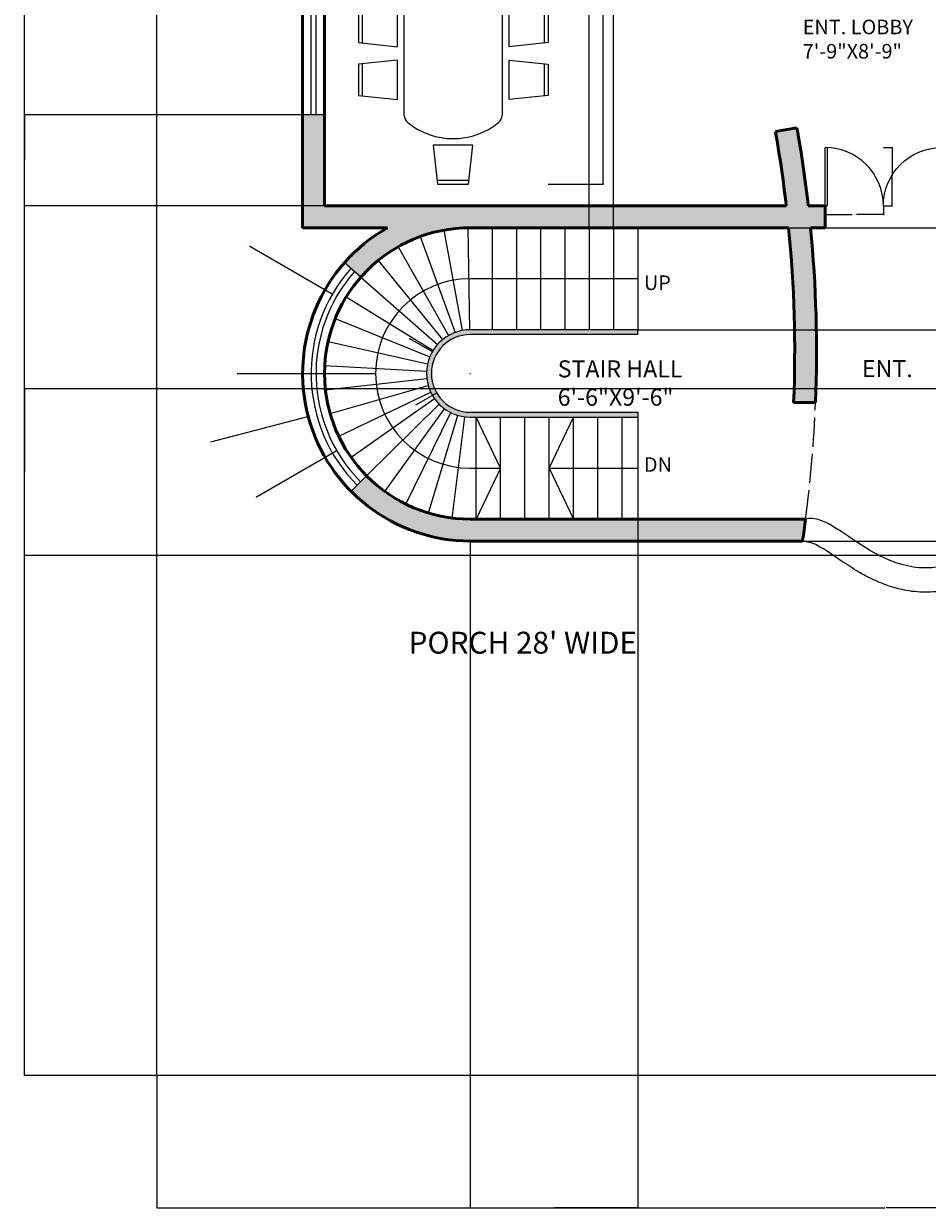
# Model space of a CAD drawing. Units: inches. Extents: x 134045 to 134755, y 144691 to 145880.
# Tile 1 of 6: x 134045 to 134417, y 144691 to 145178. Entities that reach past the tile are written whole.
import ezdxf

# ---------------------------------------------------------------- set-up
doc = ezdxf.new("R2010")
doc.units = ezdxf.units.IN
doc.linetypes.add('ACAD_ISO02W100', pattern=[15, 12, -3])
for name, color, linetype, lineweight in [('A-ANNO-DIMS', 2, 'Continuous', 18), ('A-ANNO-SYMB', 7, 'Continuous', 18), ('A-ANNO-TEXT', 7, 'Continuous', 18), ('A-AREA-IDEN', 7, 'Continuous', 18), ('A-DOOR', 4, 'Continuous', 25), ('A-FLOR-STEP', 7, 'Continuous', 25), ('A-FLOR-STRS', 7, 'Continuous', 25), ('A-FLOR-STRS-PATT', 252, 'Continuous', 13), ('A-FURN', 8, 'Continuous', 18), ('A-GLAZ', 4, 'Continuous', 18), ('A-WALL', 7, 'Continuous', 50), ('A-WALL-OVHD', 7, 'ACAD_ISO02W100', 18), ('A-WALL-PATT', 252, 'Continuous', 13), ('C-PROP', 7, 'Continuous', 25)]:
    doc.layers.add(name, color=color, linetype=linetype, lineweight=lineweight)
doc.styles.get("Standard").update_dxf_attribs({"font": 'arial.ttf'})
doc.dimstyles.get("Standard").update_dxf_attribs({"dimtxt": 0.18, "dimasz": 0.18, "dimexe": 0.18, "dimexo": 0.0625, "dimgap": 0.09, "dimtad": 0, "dimtih": 1, "dimtoh": 1, "dimdec": 4, "dimzin": 0, "dimdsep": 46, "dimtxsty": 'Standard', "dimcen": 0.09, "dimadec": 0, "dimazin": 0, "dimtfac": 1, "dimtdec": 4, "dimtofl": 0, "dimtmove": 0, "dimatfit": 3, "dimfxl": 1, "dimtolj": 1, "dimtzin": 0, "dimarcsym": 0})

# ---------------------------------------------------------------- blocks, each defined once
blk = doc.blocks.new('*U1')
blk.add_line((0, 0), (0, 42))
blk = doc.blocks.new('*U2')
at = {"layer": 'A-FLOR-STRS', "color": 0, "linetype": 'ByBlock', "lineweight": -2, "transparency": 16777216}
for p, rotation in [((134208.53, 145090.74), 200.0535228295788), ((134218.17, 145093.37), 190.5042262440651), ((134228.1, 145094.37), 180.9549296585513), ((134238.1, 145094.38), 180), ((134248.1, 145094.38), 180), ((134258.1, 145094.38), 180), ((134268.1, 145094.38), 180), ((134278.1, 145094.38), 180), ((134288.1, 145094.38), 180), ((134298.1, 145094.38), 180), ((134199.46, 145086.54), 209.6028194150926), ((134191.22, 145080.9), 219.1521160006063), ((134184.03, 145073.97), 228.70141258612), ((134178.08, 145065.95), 238.2507091716337), ((134173.55, 145057.05), 247.8000057571474), ((134170.56, 145047.52), 257.3493023426611), ((134169.19, 145037.62), 266.8985989281748), ((134169.48, 145027.64), 276.4478955136885), ((134171.43, 145017.84), 285.9971920992022), ((134174.97, 145008.5), 295.5464886847159), ((134180.01, 144999.88), 305.0957852702297), ((134186.42, 144992.21), 314.6450818557434), ((134194, 144985.71), 324.1943784412572), ((134202.56, 144980.57), 333.7436750267709), ((134211.86, 144976.91), 343.2929716122846), ((134221.63, 144974.84), 352.8422681977984)]:
    blk.add_blockref('*U1', p, dxfattribs=dict(at, rotation=rotation))
for p in [(134231.61, 144974.38), (134241.61, 144974.38), (134251.61, 144974.38), (134261.61, 144974.38), (134271.61, 144974.38), (134281.61, 144974.38), (134291.61, 144974.38)]:
    blk.add_blockref('*U1', p, dxfattribs=at)
blk = doc.blocks.new('A$C113D154D')
for p, q in [((0.96, 1.712), (1.008, 2.155)), ((1.008, 2.155), (1.362, 2.155)), ((1.362, 2.155), (1.41, 1.712)), ((1.56, 1.712), (1.608, 2.155)), ((1.608, 2.155), (1.962, 2.155)), ((1.962, 2.155), (2.01, 1.712)), ((2.16, 1.712), (2.208, 2.155)), ((2.208, 2.155), (2.562, 2.155)), ((2.562, 2.155), (2.61, 1.712)), ((2.76, 1.712), (2.808, 2.155)), ((2.808, 2.155), (3.162, 2.155)), ((3.162, 2.155), (3.21, 1.712)), ((1.003, 2.112), (1.367, 2.112)), ((1.603, 2.112), (1.967, 2.112)), ((2.203, 2.112), (2.567, 2.112)), ((2.803, 2.112), (3.167, 2.112)), ((0.78, 1.633), (3.39, 1.633)), ((1.41, 1.712), (0.96, 1.712)), ((2.01, 1.712), (1.56, 1.712)), ((2.61, 1.712), (2.16, 1.712)), ((3.21, 1.712), (2.76, 1.712)), ((0, 1.252), (0.443, 1.3)), ((0, 0.897), (0, 1.252)), ((0.043, 0.893), (0.043, 1.257)), ((0.443, 1.3), (0.443, 0.85)), ((3.727, 1.3), (3.727, 0.85)), ((4.17, 1.252), (3.727, 1.3)), ((4.127, 0.893), (4.127, 1.257)), ((4.17, 0.897), (4.17, 1.252)), ((0.443, 0.85), (0, 0.897)), ((3.727, 0.85), (4.17, 0.897)), ((3.39, 0.521), (0.78, 0.521)), ((1.41, 0.443), (0.96, 0.443)), ((0.96, 0.443), (1.008, 0)), ((1.362, 0), (1.41, 0.443)), ((2.01, 0.443), (1.56, 0.443)), ((1.56, 0.443), (1.608, 0)), ((1.962, 0), (2.01, 0.443)), ((2.61, 0.443), (2.16, 0.443)), ((2.16, 0.443), (2.208, 0)), ((2.562, 0), (2.61, 0.443)), ((3.21, 0.443), (2.76, 0.443)), ((2.76, 0.443), (2.808, 0)), ((3.162, 0), (3.21, 0.443)), ((1.003, 0.043), (1.367, 0.043)), ((1.008, 0), (1.362, 0)), ((1.603, 0.043), (1.967, 0.043)), ((1.608, 0), (1.962, 0)), ((2.203, 0.043), (2.567, 0.043)), ((2.208, 0), (2.562, 0)), ((2.803, 0.043), (3.167, 0.043)), ((2.808, 0), (3.162, 0))]:
    blk.add_line(p, q)
for centre, radius, start, end in [((0.78, 1.533), 0.1, 90, 140.3976), ((3.39, 1.533), 0.1, 39.6024, 90), ((1.331, 1.077), 0.815, 140.3976, 219.6024), ((2.839, 1.077), 0.815, 320.3976, 39.6024), ((0.78, 0.621), 0.1, 219.6024, 270), ((3.39, 0.621), 0.1, 270, 320.3976)]:
    blk.add_arc(centre, radius, start, end)
blk = doc.blocks.new('DOOR-SWING-24IN')
for p, q in [((0, 0), (0, 24)), ((1, 0), (1, 23.98)), ((1, 0), (0, 0))]:
    blk.add_line(p, q)
blk.add_arc((0, 0), 24, 0, 90)
blk = doc.blocks.new('WIN-GLAZ-96IN')
for p, q in [((0, 0), (0, 96)), ((2, 0), (2, 96))]:
    blk.add_line(p, q)
blk = doc.blocks.new('*D24')
at = {"layer": 'A-ANNO-DIMS', "color": 0, "lineweight": -2, "transparency": 16777216}
for p, q in [((134375.19, 145103.31), (134375.19, 145099.6)), ((134375.37, 145099.78), (134386.32, 145099.78)), ((134399.01, 145099.78), (134388.07, 145099.78)), ((134399.19, 145103.31), (134399.19, 145099.6))]:
    blk.add_line(p, q, dxfattribs=at)
at = {"layer": 'A-ANNO-DIMS', "color": 0, "transparency": 16777216}
for points in [[(134375.37, 145099.81), (134375.37, 145099.75), (134375.19, 145099.78)], [(134399.01, 145099.81), (134399.01, 145099.75), (134399.19, 145099.78)]]:
    blk.add_solid(points, dxfattribs=at)
at = {"layer": 'Defpoints', "color": 0, "transparency": 16777216}
for p in [(134375.19, 145103.38), (134399.19, 145103.38), (134399.19, 145099.78)]:
    blk.add_point(p, dxfattribs=at)
at = {"layer": 'A-ANNO-DIMS', "color": 0, "transparency": 16777216, "insert": (134387.19, 145099.78), "char_height": 0.18, "attachment_point": 5}
blk.add_mtext('\\A1;LEAF 24 TYP.', dxfattribs=at)
blk = doc.blocks.new('*D25')
at = {"layer": 'A-ANNO-DIMS', "color": 0, "lineweight": -2, "transparency": 16777216}
for p, q in [((134399.26, 145127.38), (134402.97, 145127.38)), ((134402.79, 145127.2), (134402.79, 145115.56)), ((134402.79, 145103.56), (134402.79, 145115.19)), ((134399.26, 145103.38), (134402.97, 145103.38))]:
    blk.add_line(p, q, dxfattribs=at)
at = {"layer": 'A-ANNO-DIMS', "color": 0, "transparency": 16777216}
for points in [[(134402.76, 145127.2), (134402.82, 145127.2), (134402.79, 145127.38)], [(134402.76, 145103.56), (134402.82, 145103.56), (134402.79, 145103.38)]]:
    blk.add_solid(points, dxfattribs=at)
at = {"layer": 'Defpoints', "color": 0, "transparency": 16777216}
for p in [(134399.19, 145127.38), (134402.79, 145127.38), (134399.19, 145103.38)]:
    blk.add_point(p, dxfattribs=at)
at = {"layer": 'A-ANNO-DIMS', "color": 0, "transparency": 16777216, "insert": (134402.79, 145115.38), "char_height": 0.18, "attachment_point": 5}
blk.add_mtext('\\A1;24 TYP.', dxfattribs=at)
blk = doc.blocks.new('*D40')
at = {"layer": 'A-ANNO-DIMS', "color": 0, "lineweight": -2, "transparency": 16777216}
for p, q in [((134261.18, 145263.4), (134283.96, 145263.4)), ((134283.78, 145263.22), (134283.78, 145188.06)), ((134283.78, 145112.53), (134283.78, 145187.69)), ((134261.18, 145112.35), (134283.96, 145112.35))]:
    blk.add_line(p, q, dxfattribs=at)
at = {"layer": 'A-ANNO-DIMS', "color": 0, "transparency": 16777216}
for points in [[(134283.75, 145263.22), (134283.81, 145263.22), (134283.78, 145263.4)], [(134283.75, 145112.53), (134283.81, 145112.53), (134283.78, 145112.35)]]:
    blk.add_solid(points, dxfattribs=at)
at = {"layer": 'Defpoints', "color": 0, "transparency": 16777216}
for p in [(134261.12, 145263.4), (134261.12, 145112.35), (134283.78, 145112.35)]:
    blk.add_point(p, dxfattribs=at)
at = {"layer": 'A-ANNO-DIMS', "color": 0, "transparency": 16777216, "insert": (134283.78, 145187.88), "char_height": 0.18, "attachment_point": 5}
blk.add_mtext('\\A1;DINING SET 151', dxfattribs=at)
blk = doc.blocks.new('*D46')
at = {"layer": 'A-ANNO-DIMS', "color": 0, "lineweight": -2, "transparency": 16777216}
for p, q in [((134100.1, 144745.31), (134100.1, 144690.65)), ((134700.1, 144745.31), (134700.1, 144690.65)), ((134100.28, 144690.83), (134399.81, 144690.83)), ((134699.92, 144690.83), (134400.39, 144690.83))]:
    blk.add_line(p, q, dxfattribs=at)
at = {"layer": 'A-ANNO-DIMS', "color": 0, "transparency": 16777216}
for points in [[(134100.28, 144690.86), (134100.28, 144690.8), (134100.1, 144690.83)], [(134699.92, 144690.86), (134699.92, 144690.8), (134700.1, 144690.83)]]:
    blk.add_solid(points, dxfattribs=at)
at = {"layer": 'Defpoints', "color": 0, "transparency": 16777216}
for p in [(134100.1, 144745.38), (134700.1, 144745.38), (134700.1, 144690.83)]:
    blk.add_point(p, dxfattribs=at)
at = {"layer": 'A-ANNO-DIMS', "color": 0, "transparency": 16777216, "insert": (134400.1, 144690.83), "char_height": 0.18, "attachment_point": 5}
blk.add_mtext('\\A1;600', dxfattribs=at)
blk = doc.blocks.new('*D47')
at = {"layer": 'A-ANNO-DIMS', "color": 0, "lineweight": -2, "transparency": 16777216}
for p, q in [((134100.04, 145825.38), (134045.37, 145825.38)), ((134045.55, 145825.2), (134045.55, 145285.56)), ((134045.55, 144745.56), (134045.55, 145285.19)), ((134100.04, 144745.38), (134045.37, 144745.38))]:
    blk.add_line(p, q, dxfattribs=at)
at = {"layer": 'A-ANNO-DIMS', "color": 0, "transparency": 16777216}
for points in [[(134045.52, 145825.2), (134045.58, 145825.2), (134045.55, 145825.38)], [(134045.52, 144745.56), (134045.58, 144745.56), (134045.55, 144745.38)]]:
    blk.add_solid(points, dxfattribs=at)
at = {"layer": 'Defpoints', "color": 0, "transparency": 16777216}
for p in [(134045.55, 145825.38), (134100.1, 145825.38), (134100.1, 144745.38)]:
    blk.add_point(p, dxfattribs=at)
at = {"layer": 'A-ANNO-DIMS', "color": 0, "transparency": 16777216, "insert": (134045.55, 145285.38), "char_height": 0.18, "attachment_point": 5}
blk.add_mtext('\\A1;1080', dxfattribs=at)
blk = doc.blocks.new('*D54')
at = {"layer": 'A-ANNO-DIMS', "color": 0, "lineweight": -2, "transparency": 16777216}
for p, q in [((134298.1, 144974.31), (134298.1, 144690.65)), ((134229.1, 144965.31), (134229.1, 144690.65)), ((134229.28, 144690.83), (134263.38, 144690.83)), ((134297.92, 144690.83), (134263.82, 144690.83))]:
    blk.add_line(p, q, dxfattribs=at)
at = {"layer": 'A-ANNO-DIMS', "color": 0, "transparency": 16777216}
for points in [[(134229.28, 144690.86), (134229.28, 144690.8), (134229.1, 144690.83)], [(134297.92, 144690.86), (134297.92, 144690.8), (134298.1, 144690.83)]]:
    blk.add_solid(points, dxfattribs=at)
at = {"layer": 'Defpoints', "color": 0, "transparency": 16777216}
for p in [(134298.1, 144974.38), (134229.1, 144965.38), (134298.1, 144690.83)]:
    blk.add_point(p, dxfattribs=at)
at = {"layer": 'A-ANNO-DIMS', "color": 0, "transparency": 16777216, "insert": (134263.6, 144690.83), "char_height": 0.18, "attachment_point": 5}
blk.add_mtext('\\A1;69', dxfattribs=at)
blk = doc.blocks.new('*D55')
at = {"layer": 'A-ANNO-DIMS', "color": 0, "lineweight": -2, "transparency": 16777216}
for p, q in [((134278.1, 145094.44), (134278.1, 145880.11)), ((134288.1, 145094.44), (134288.1, 145880.11)), ((134278.28, 145879.93), (134282.89, 145879.93)), ((134287.92, 145879.93), (134283.31, 145879.93))]:
    blk.add_line(p, q, dxfattribs=at)
at = {"layer": 'A-ANNO-DIMS', "color": 0, "transparency": 16777216}
for points in [[(134278.28, 145879.96), (134278.28, 145879.9), (134278.1, 145879.93)], [(134287.92, 145879.96), (134287.92, 145879.9), (134288.1, 145879.93)]]:
    blk.add_solid(points, dxfattribs=at)
at = {"layer": 'Defpoints', "color": 0, "transparency": 16777216}
for p in [(134288.1, 145879.93), (134278.1, 145094.38), (134288.1, 145094.38)]:
    blk.add_point(p, dxfattribs=at)
at = {"layer": 'A-ANNO-DIMS', "color": 0, "transparency": 16777216, "insert": (134283.1, 145879.93), "char_height": 0.18, "attachment_point": 5}
blk.add_mtext('\\A1;10', dxfattribs=at)
blk = doc.blocks.new('*D56')
at = {"layer": 'A-ANNO-DIMS', "color": 0, "lineweight": -2, "transparency": 16777216}
for p, q in [((134298.17, 145094.38), (134754.83, 145094.38)), ((134754.65, 145094.2), (134754.65, 145073.56)), ((134754.65, 145052.56), (134754.65, 145073.19)), ((134298.17, 145052.38), (134754.83, 145052.38))]:
    blk.add_line(p, q, dxfattribs=at)
at = {"layer": 'A-ANNO-DIMS', "color": 0, "transparency": 16777216}
for points in [[(134754.62, 145094.2), (134754.68, 145094.2), (134754.65, 145094.38)], [(134754.62, 145052.56), (134754.68, 145052.56), (134754.65, 145052.38)]]:
    blk.add_solid(points, dxfattribs=at)
at = {"layer": 'Defpoints', "color": 0, "transparency": 16777216}
for p in [(134298.1, 145094.38), (134754.65, 145094.38), (134298.1, 145052.38)]:
    blk.add_point(p, dxfattribs=at)
at = {"layer": 'A-ANNO-DIMS', "color": 0, "transparency": 16777216, "insert": (134754.65, 145073.38), "char_height": 0.18, "attachment_point": 5}
blk.add_mtext('\\A1;42', dxfattribs=at)
blk = doc.blocks.new('*D65')
at = {"layer": 'A-ANNO-DIMS', "color": 0, "lineweight": -2, "transparency": 16777216}
for p, q in [((134365.99, 144965.38), (134754.83, 144965.38)), ((134754.65, 144965.2), (134754.65, 144958.06)), ((134754.65, 144950.56), (134754.65, 144957.69)), ((134430.17, 144950.38), (134754.83, 144950.38))]:
    blk.add_line(p, q, dxfattribs=at)
at = {"layer": 'A-ANNO-DIMS', "color": 0, "transparency": 16777216}
for points in [[(134754.62, 144965.2), (134754.68, 144965.2), (134754.65, 144965.38)], [(134754.62, 144950.56), (134754.68, 144950.56), (134754.65, 144950.38)]]:
    blk.add_solid(points, dxfattribs=at)
at = {"layer": 'Defpoints', "color": 0, "transparency": 16777216}
for p in [(134365.92, 144965.38), (134754.65, 144965.38), (134430.1, 144950.38)]:
    blk.add_point(p, dxfattribs=at)
at = {"layer": 'A-ANNO-DIMS', "color": 0, "transparency": 16777216, "insert": (134754.65, 144957.88), "char_height": 0.18, "attachment_point": 5}
blk.add_mtext('\\A1;15', dxfattribs=at)
blk = doc.blocks.new('*D67')
at = {"layer": 'A-ANNO-DIMS', "color": 0, "lineweight": -2, "transparency": 16777216}
for p, q in [((134439.04, 145028.04), (134045.37, 145028.04)), ((134045.55, 145027.86), (134045.55, 144993.89)), ((134045.55, 144959.56), (134045.55, 144993.53)), ((134439.04, 144959.38), (134045.37, 144959.38))]:
    blk.add_line(p, q, dxfattribs=at)
at = {"layer": 'A-ANNO-DIMS', "color": 0, "transparency": 16777216}
for points in [[(134045.52, 145027.86), (134045.58, 145027.86), (134045.55, 145028.04)], [(134045.52, 144959.56), (134045.58, 144959.56), (134045.55, 144959.38)]]:
    blk.add_solid(points, dxfattribs=at)
at = {"layer": 'Defpoints', "color": 0, "transparency": 16777216}
for p in [(134045.55, 145028.04), (134439.1, 145028.04), (134439.1, 144959.38)]:
    blk.add_point(p, dxfattribs=at)
at = {"layer": 'A-ANNO-DIMS', "color": 0, "transparency": 16777216, "insert": (134045.55, 144993.71), "char_height": 0.18, "attachment_point": 5}
blk.add_mtext('\\A1;68.66', dxfattribs=at)
blk = doc.blocks.new('*D74')
at = {"layer": 'A-ANNO-DIMS', "color": 0, "lineweight": -2, "transparency": 16777216}
for p, q in [((134169.04, 145140.88), (134045.37, 145140.88)), ((134045.55, 145140.7), (134045.55, 145122.31)), ((134045.55, 145103.56), (134045.55, 145121.94)), ((134169.04, 145103.38), (134045.37, 145103.38))]:
    blk.add_line(p, q, dxfattribs=at)
at = {"layer": 'A-ANNO-DIMS', "color": 0, "transparency": 16777216}
for points in [[(134045.52, 145140.7), (134045.58, 145140.7), (134045.55, 145140.88)], [(134045.52, 145103.56), (134045.58, 145103.56), (134045.55, 145103.38)]]:
    blk.add_solid(points, dxfattribs=at)
at = {"layer": 'Defpoints', "color": 0, "transparency": 16777216}
for p in [(134045.55, 145140.88), (134169.1, 145140.88), (134169.1, 145103.38)]:
    blk.add_point(p, dxfattribs=at)
at = {"layer": 'A-ANNO-DIMS', "color": 0, "transparency": 16777216, "insert": (134045.55, 145122.13), "char_height": 0.18, "attachment_point": 5}
blk.add_mtext('\\A1;37.5', dxfattribs=at)
blk = doc.blocks.new('*D76')
at = {"layer": 'A-ANNO-DIMS', "color": 0, "lineweight": -2, "transparency": 16777216}
for p, q in [((134229.01, 145034.38), (134229.19, 145034.38)), ((134229.1, 145034.29), (134229.1, 145034.47)), ((134122.36, 145006.18), (134162.22, 145016.71))]:
    blk.add_line(p, q, dxfattribs=at)
at = {"layer": 'A-ANNO-DIMS', "color": 0, "transparency": 16777216}
blk.add_solid([(134162.21, 145016.74), (134162.23, 145016.68), (134162.39, 145016.75)], dxfattribs=at)
at = {"layer": 'Defpoints', "color": 0, "transparency": 16777216}
for p in [(134229.1, 145034.38), (134162.39, 145016.75)]:
    blk.add_point(p, dxfattribs=at)
at = {"layer": 'A-ANNO-DIMS', "color": 0, "transparency": 16777216, "insert": (134122.06, 145006.18), "char_height": 0.18, "attachment_point": 5}
blk.add_mtext('\\A1;R69', dxfattribs=at)
blk = doc.blocks.new('*D77')
at = {"layer": 'A-ANNO-DIMS', "color": 0, "lineweight": -2, "transparency": 16777216}
for p, q in [((134138.16, 145086.78), (134138.34, 145086.78)), ((134138.34, 145086.78), (134172.22, 145067.22)), ((134229.01, 145034.38), (134229.19, 145034.38)), ((134229.1, 145034.29), (134229.1, 145034.47))]:
    blk.add_line(p, q, dxfattribs=at)
at = {"layer": 'A-ANNO-DIMS', "color": 0, "transparency": 16777216}
blk.add_solid([(134172.24, 145067.24), (134172.21, 145067.19), (134172.38, 145067.13)], dxfattribs=at)
at = {"layer": 'Defpoints', "color": 0, "transparency": 16777216}
for p in [(134172.38, 145067.13), (134229.1, 145034.38)]:
    blk.add_point(p, dxfattribs=at)
at = {"layer": 'A-ANNO-DIMS', "color": 0, "transparency": 16777216, "insert": (134137.75, 145086.78), "char_height": 0.18, "attachment_point": 5}
blk.add_mtext('\\A1;R65.5', dxfattribs=at)
blk = doc.blocks.new('*D78')
at = {"layer": 'A-ANNO-DIMS', "color": 0, "lineweight": -2, "transparency": 16777216}
for p, q in [((134229.01, 145034.38), (134229.19, 145034.38)), ((134229.1, 145034.29), (134229.1, 145034.47)), ((134141.12, 144983.58), (134173.96, 145002.54)), ((134140.94, 144983.58), (134141.12, 144983.58))]:
    blk.add_line(p, q, dxfattribs=at)
at = {"layer": 'A-ANNO-DIMS', "color": 0, "transparency": 16777216}
blk.add_solid([(134173.94, 145002.56), (134173.97, 145002.51), (134174.11, 145002.63)], dxfattribs=at)
at = {"layer": 'Defpoints', "color": 0, "transparency": 16777216}
for p in [(134229.1, 145034.38), (134174.11, 145002.63)]:
    blk.add_point(p, dxfattribs=at)
at = {"layer": 'A-ANNO-DIMS', "color": 0, "transparency": 16777216, "insert": (134140.52, 144983.58), "char_height": 0.18, "attachment_point": 5}
blk.add_mtext('\\A1;R63.5', dxfattribs=at)
blk = doc.blocks.new('*D79')
at = {"layer": 'A-ANNO-DIMS', "color": 0, "lineweight": -2, "transparency": 16777216}
for p, q in [((134133.1, 145034.37), (134168.92, 145034.37)), ((134229.01, 145034.38), (134229.19, 145034.38)), ((134229.1, 145034.29), (134229.1, 145034.47))]:
    blk.add_line(p, q, dxfattribs=at)
at = {"layer": 'A-ANNO-DIMS', "color": 0, "transparency": 16777216}
blk.add_solid([(134168.92, 145034.4), (134168.92, 145034.34), (134169.1, 145034.37)], dxfattribs=at)
at = {"layer": 'Defpoints', "color": 0, "transparency": 16777216}
for p in [(134169.1, 145034.37), (134229.1, 145034.38)]:
    blk.add_point(p, dxfattribs=at)
at = {"layer": 'A-ANNO-DIMS', "color": 0, "transparency": 16777216, "insert": (134132.8, 145034.37), "char_height": 0.18, "attachment_point": 5}
blk.add_mtext('\\A1;R60', dxfattribs=at)
blk = doc.blocks.new('*D80')
at = {"layer": 'A-ANNO-DIMS', "color": 0, "lineweight": -2, "transparency": 16777216}
for p, q in [((134203.98, 145048.78), (134204.16, 145048.78)), ((134204.16, 145048.78), (134213.36, 145043.47)), ((134229.01, 145034.38), (134229.19, 145034.38)), ((134229.1, 145034.29), (134229.1, 145034.47))]:
    blk.add_line(p, q, dxfattribs=at)
at = {"layer": 'A-ANNO-DIMS', "color": 0, "transparency": 16777216}
blk.add_solid([(134213.37, 145043.49), (134213.34, 145043.44), (134213.52, 145043.38)], dxfattribs=at)
at = {"layer": 'Defpoints', "color": 0, "transparency": 16777216}
for p in [(134213.52, 145043.38), (134229.1, 145034.38)]:
    blk.add_point(p, dxfattribs=at)
at = {"layer": 'A-ANNO-DIMS', "color": 0, "transparency": 16777216, "insert": (134203.68, 145048.78), "char_height": 0.18, "attachment_point": 5}
blk.add_mtext('\\A1;R18', dxfattribs=at)
blk = doc.blocks.new('*D81')
at = {"layer": 'A-ANNO-DIMS', "color": 0, "lineweight": -2, "transparency": 16777216}
for p, q in [((134229.01, 145034.38), (134229.19, 145034.38)), ((134229.1, 145034.29), (134229.1, 145034.47)), ((134206.93, 145021.57), (134215.09, 145026.28)), ((134206.75, 145021.57), (134206.93, 145021.57))]:
    blk.add_line(p, q, dxfattribs=at)
at = {"layer": 'A-ANNO-DIMS', "color": 0, "transparency": 16777216}
blk.add_solid([(134215.08, 145026.31), (134215.11, 145026.26), (134215.25, 145026.37)], dxfattribs=at)
at = {"layer": 'Defpoints', "color": 0, "transparency": 16777216}
for p in [(134229.1, 145034.38), (134215.25, 145026.37)]:
    blk.add_point(p, dxfattribs=at)
at = {"layer": 'A-ANNO-DIMS', "color": 0, "transparency": 16777216, "insert": (134206.45, 145021.57), "char_height": 0.18, "attachment_point": 5}
blk.add_mtext('\\A1;R16', dxfattribs=at)
blk = doc.blocks.new('*D82')
at = {"layer": 'A-ANNO-DIMS', "color": 0, "lineweight": -2, "transparency": 16777216}
for p, q in [((134166.7, 145034.37), (134189.92, 145034.37)), ((134229.01, 145034.38), (134229.19, 145034.38)), ((134229.1, 145034.29), (134229.1, 145034.47))]:
    blk.add_line(p, q, dxfattribs=at)
at = {"layer": 'A-ANNO-DIMS', "color": 0, "transparency": 16777216}
blk.add_solid([(134189.92, 145034.4), (134189.92, 145034.34), (134190.1, 145034.37)], dxfattribs=at)
at = {"layer": 'Defpoints', "color": 0, "transparency": 16777216}
for p in [(134190.1, 145034.37), (134229.1, 145034.38)]:
    blk.add_point(p, dxfattribs=at)
at = {"layer": 'A-ANNO-DIMS', "color": 0, "transparency": 16777216, "insert": (134166.4, 145034.37), "char_height": 0.18, "attachment_point": 5}
blk.add_mtext('\\A1;R39', dxfattribs=at)

msp = doc.modelspace()

# ---------------------------------------------------------------- hatches: boundary and pattern name
at = {"layer": 'A-FLOR-STRS-PATT'}
h = msp.add_hatch(color=256, dxfattribs=at)
h.dxf.hatch_style = 1
h.paths.add_polyline_path([(134229.1037, 145050.3753), (134298.1037, 145050.3753), (134298.1037, 145052.3753), (134229.1037, 145052.3753, 1), (134229.1037, 145016.3753), (134298.1037, 145016.3753), (134298.1037, 145018.3753), (134229.1037, 145018.3753, -1)])
at = {"layer": 'A-WALL-PATT'}
h = msp.add_hatch(color=256, dxfattribs=at)
h.dxf.hatch_style = 1
h.paths.add_polyline_path([(134367.1819, 144974.3753), (134298.1037, 144974.3753), (134229.1037, 144974.3753, -0.20052276), (134186.4153, 144992.2125), (134180.012, 144985.8881, 0.20052276), (134229.1037, 144965.3753), (134365.9246, 144965.3753, 0.00427598)])
h.paths.add_polyline_path([(134375.1948, 145103.3753), (134368.2859, 145103.3753, 0.01529186), (134363.6321, 145135.5319), (134354.7685, 145133.9711, -0.01480221), (134359.227, 145103.3753), (134169.1037, 145103.3753), (134169.1037, 145140.8753), (134160.1037, 145140.8753), (134160.1037, 145094.3753), (134195.0303, 145094.3753, 0.08357499), (134177.2654, 145079.9142), (134184.0269, 145073.9743, -0.21575742), (134229.1037, 145094.3753), (134298.1037, 145094.3753), (134360.1885, 145094.3753, -0.03451726), (134362.2602, 145022.3753), (134371.2674, 145022.3753, 0.03393073), (134369.231, 145094.3753), (134375.1948, 145094.3753)])

# ---------------------------------------------------------------- linework, layer by layer
at = {"layer": 'A-ANNO-SYMB'}
for p, q in [((134241.6082, 144995.3753), (134231.6082, 145016.3753)), ((134261.6082, 144995.3753), (134271.6082, 145016.3753)), ((134241.6082, 144995.3753), (134231.6082, 144974.3753)), ((134261.6082, 144995.3753), (134271.6082, 144974.3753))]:
    msp.add_line(p, q, dxfattribs=at)
msp.add_lwpolyline([(134298.1037, 145073.3753), (134229.1037, 145073.3753, 1), (134229.1037, 144995.3753), (134241.6082, 144995.3753)], format="xyb", dxfattribs=at)
msp.add_lwpolyline([(134261.6082, 144995.3753), (134298.1037, 144995.3753)], dxfattribs=at)
at = {"layer": 'A-FLOR-STEP'}
msp.add_open_spline([(134430.1037, 144957.0094), (134399.3308, 144944.8123), (134380.3033, 144978.1647), (134367.1819, 144974.3753)], degree=3, dxfattribs=at)
msp.add_open_spline([(134437.1757, 144950.3753), (134431.726, 144946.8956), (134429.6738, 144946.2317), (134424.5415, 144944.9303), (134421.4861, 144944.4905), (134415.5549, 144944.2239), (134412.6813, 144944.3964), (134407.1936, 144945.2148), (134404.5797, 144945.8591), (134399.6343, 144947.459), (134397.3016, 144948.4141), (134392.9017, 144950.4905), (134390.8335, 144951.612), (134386.3854, 144954.2214), (134384.0816, 144955.7235), (134379.8453, 144958.5591), (134377.9107, 144959.8932), (134375.0049, 144961.8012), (134373.9221, 144962.4818), (134372.0202, 144963.5793), (134371.2004, 144963.9937), (134370.0661, 144964.4771), (134369.6889, 144964.5945), (134365.9246, 144965.3753)], degree=3, knots=[0, 0, 0, 0, 0.49462993, 0.49462993, 1.24835968, 1.24835968, 2.00208942, 2.00208942, 2.75581917, 2.75581917, 3.50954892, 3.50954892, 4.26327867, 4.26327867, 5.23068651, 5.23068651, 6.19809434, 6.19809434, 6.86222056, 6.86222056, 7.52634677, 7.52634677, 8.06757639, 8.06757639, 8.06757639, 8.06757639], dxfattribs=at)
at = {"layer": 'A-FLOR-STRS'}
for p, q in [((134298.1037, 145050.3753), (134298.1037, 145052.3753)), ((134298.1037, 145018.3753), (134298.1037, 144974.3753))]:
    msp.add_line(p, q, dxfattribs=at)
for points in [[(134298.1037, 145052.3753), (134229.1037, 145052.3753, 1), (134229.1037, 145016.3753), (134298.1037, 145016.3753)], [(134298.1037, 145050.3753), (134229.1037, 145050.3753, 1), (134229.1037, 145018.3753), (134298.1037, 145018.3753)]]:
    msp.add_lwpolyline(points, format="xyb", dxfattribs=at)
at = {"layer": 'A-GLAZ'}
for p, q in [((134169.1037, 145140.8753), (134160.1037, 145140.8753)), ((134184.0269, 145073.9743), (134177.2654, 145079.9142)), ((134186.4153, 144992.2125), (134180.012, 144985.8881))]:
    msp.add_line(p, q, dxfattribs=at)
for radius in [65.5, 63.5]:
    msp.add_arc((134229.1037, 145034.3753), radius, 138.701413, 224.645082, dxfattribs=at)
at = {"layer": 'A-WALL'}
for p, q in [((134160.1037, 145094.3753), (134160.1037, 145765.3753)), ((134169.1037, 145103.3753), (134169.1037, 145274.3753)), ((134354.7685, 145133.9711), (134363.6321, 145135.5319)), ((134169.1037, 145103.3753), (134359.227, 145103.3753)), ((134368.2859, 145103.3753), (134375.1948, 145103.3753)), ((134375.1948, 145103.3753), (134375.1948, 145094.3753)), ((134160.1037, 145094.3753), (134195.0303, 145094.3753)), ((134369.231, 145094.3753), (134375.1948, 145094.3753)), ((134229.1037, 144965.3753), (134365.9246, 144965.3753))]:
    msp.add_line(p, q, dxfattribs=at)
msp.add_lwpolyline([(134298.1037, 145094.3753), (134229.1037, 145094.3753, 1), (134229.1037, 144974.3753), (134298.1037, 144974.3753)], format="xyb", dxfattribs=at)
for points in [[(134360.1885, 145094.3753), (134298.1037, 145094.3753)], [(134362.2602, 145022.3753), (134371.2674, 145022.3753)], [(134298.1037, 144974.3753), (134367.1819, 144974.3753)]]:
    msp.add_lwpolyline(points, dxfattribs=at)
for centre, radius, start, end in [((133840.3674, 145043.3884), 522.3157, 6.594858, 9.987027), ((133840.3674, 145043.3884), 531.3157, 6.482664, 9.987027), ((134229.1037, 145034.3753), 69, 119.591846, 270), ((133840.3674, 145043.3884), 522.3157, 357.694333, 5.601966), ((133840.3674, 145043.3884), 531.3157, 357.736806, 5.506778), ((133840.3674, 145043.3884), 531.3157, 351.556735, 352.536711)]:
    msp.add_arc(centre, radius, start, end, dxfattribs=at)
at = {"layer": 'A-WALL-OVHD'}
msp.add_arc((133840.3674, 145043.3884), 531.3157, 352.536711, 357.736806, dxfattribs=at)
at = {"layer": 'C-PROP'}
for p, q in [((134100.1037, 144745.3753), (134100.1037, 145825.3753)), ((134700.1037, 144745.3753), (134100.1037, 144745.3753))]:
    msp.add_line(p, q, dxfattribs=at)

# ---------------------------------------------------------------- block references
at = {"layer": 'A-DOOR'}
msp.add_blockref('DOOR-SWING-24IN', (134375.195, 145103.375), dxfattribs=at)
at = {"layer": 'A-DOOR', "extrusion": (0, 0, -1), "zscale": -1}
msp.add_blockref('DOOR-SWING-24IN', (-134423.1946, 145103.375), dxfattribs=at)
at = {"layer": 'A-FLOR-STRS'}
msp.add_blockref('*U2', (0, 0), dxfattribs=at)
at = {"layer": 'A-FURN', "xscale": 36.22436829030262, "yscale": 36.22436829030262, "zscale": 36.22436829030262, "rotation": 270}
msp.add_blockref('A$C113D154D', (134183.0679, 145263.4031), dxfattribs=at)
at = {"layer": 'A-GLAZ'}
msp.add_blockref('WIN-GLAZ-96IN', (134163.604, 145140.875), dxfattribs=at)

# ---------------------------------------------------------------- texts
at = {"layer": 'A-ANNO-TEXT', "char_height": 6, "attachment_point": 1}
for s, insert in [('UP', (134300.6069, 145074.7139)), ('DN', (134300.6069, 144999.8682))]:
    msp.add_mtext_dynamic_manual_height_columns(s, width=19.204789, gutter_width=12.5, heights=[0], dxfattribs=dict(at, insert=insert))
at = {"layer": 'A-AREA-IDEN', "attachment_point": 1}
for s, width, insert, char_height in [('ENT. LOBBY\\P7\'-9"X8\'-9"', 198.060459, (134366.0069, 145180.0217), 6), ('STAIR HALL\\P6\'-6"X9\'-6"', 59.911918, (134265.1213, 145039.7574), 7), ('ENT.', 20.723753, (134390.3727, 145039.8726), 7), ("PORCH 28' WIDE", 104.726732, (134203.7214, 144928.0109), 9)]:
    msp.add_mtext_dynamic_manual_height_columns(s, width=width, gutter_width=12.5, heights=[0], dxfattribs=dict(at, insert=insert, char_height=char_height))

# ---------------------------------------------------------------- dimensions: what is measured, and where the dimension line sits
at = {"layer": 'A-ANNO-DIMS'}
for base, p1, p2, picture, middle in [((134288.1037, 145879.9253), (134278.1037, 145094.3753), (134288.1037, 145094.3753), '*D55', (134283.1037, 145879.9253)), ((134298.1037, 144690.8253), (134229.1037, 144965.3753), (134298.1037, 144974.3753), '*D54', (134263.6037, 144690.8253)), ((134700.1037, 144690.8253), (134100.1037, 144745.3753), (134700.1037, 144745.3753), '*D46', (134400.1037, 144690.8253))]:
    dim = msp.add_linear_dim(base=base, p1=p1, p2=p2, dimstyle='Standard', override={"dimdec": 0, "dimlfac": 1, "dimrnd": 0, "dimzin": 0, "dimdsep": 46, "dimlunit": 2}, dxfattribs=at)
    dim.commit()
    dim.dimension.update_dxf_attribs({"geometry": picture, "text_midpoint": middle})
for base, p1, p2, override, picture, middle in [((134045.5537, 145825.3753), (134100.1037, 144745.3753), (134100.1037, 145825.3753), {"dimdec": 0, "dimlfac": 1, "dimrnd": 0, "dimzin": 0, "dimdsep": 46, "dimlunit": 2}, '*D47', (134045.5537, 145285.3753)), ((134045.5537, 145140.8753), (134169.1037, 145103.3753), (134169.1037, 145140.8753), {"dimdec": 1, "dimlfac": 1, "dimrnd": 0, "dimzin": 0, "dimdsep": 46, "dimlunit": 2}, '*D74', (134045.5537, 145122.1253)), ((134754.6537, 145094.3753), (134298.1037, 145052.3753), (134298.1037, 145094.3753), {"dimdec": 0, "dimlfac": 1, "dimrnd": 0, "dimzin": 0, "dimdsep": 46, "dimlunit": 2}, '*D56', (134754.6537, 145073.3753)), ((134045.5537, 145028.0394), (134439.1037, 144959.3753), (134439.1037, 145028.0394), {"dimdec": 2, "dimlfac": 1, "dimrnd": 0, "dimzin": 0, "dimdsep": 46, "dimlunit": 2}, '*D67', (134045.5537, 144993.7074)), ((134754.6537, 144965.3753), (134430.1037, 144950.3753), (134365.9246, 144965.3753), {"dimdec": 0, "dimlfac": 1, "dimrnd": 0, "dimzin": 0, "dimdsep": 46, "dimlunit": 2}, '*D65', (134754.6537, 144957.8753))]:
    dim = msp.add_linear_dim(base=base, p1=p1, p2=p2, angle=90, dimstyle='Standard', override=override, dxfattribs=at)
    dim.commit()
    dim.dimension.update_dxf_attribs({"geometry": picture, "text_midpoint": middle})
for base, p1, p2, angle, text, picture, middle in [((134283.7794, 145112.3471), (134261.121, 145263.4031), (134261.121, 145112.3471), 270, 'DINING SET <>', '*D40', (134283.7794, 145187.8751)), ((134402.7948, 145127.3753), (134399.1948, 145103.3753), (134399.1948, 145127.3753), 90, '<> TYP.', '*D25', (134402.7948, 145115.3753))]:
    dim = msp.add_linear_dim(base=base, p1=p1, p2=p2, angle=angle, text=text, dimstyle='Standard', override={"dimdec": 0, "dimlfac": 1, "dimrnd": 0, "dimzin": 0, "dimdsep": 46, "dimlunit": 2}, dxfattribs=at)
    dim.commit()
    dim.dimension.update_dxf_attribs({"geometry": picture, "text_midpoint": middle})
dim = msp.add_linear_dim(base=(134399.1948, 145099.7753), p1=(134375.1948, 145103.3753), p2=(134399.1948, 145103.3753), text='LEAF <> TYP.', dimstyle='Standard', override={"dimdec": 0, "dimlfac": 1, "dimrnd": 0, "dimzin": 0, "dimdsep": 46, "dimlunit": 2}, dxfattribs=at)
dim.commit()
dim.dimension.update_dxf_attribs({"geometry": '*D24', "text_midpoint": (134387.1948, 145099.7753)})
for mpoint, override, picture, middle in [((134172.3791, 145067.1255), {"dimdec": 1, "dimlfac": 1, "dimrnd": 0, "dimzin": 0, "dimdsep": 46, "dimlunit": 2}, '*D77', (134137.7538, 145086.7756)), ((134213.5153, 145043.3754), {"dimdec": 0, "dimlfac": 1, "dimrnd": 0, "dimzin": 0, "dimdsep": 46, "dimlunit": 2}, '*D80', (134203.677, 145048.7755)), ((134162.3917, 145016.7539), {"dimdec": 0, "dimlfac": 1, "dimrnd": 0, "dimzin": 0, "dimdsep": 46, "dimlunit": 2}, '*D76', (134122.3646, 145006.1811)), ((134169.1037, 145034.375), {"dimdec": 0, "dimlfac": 1, "dimrnd": 0, "dimzin": 0, "dimdsep": 46, "dimlunit": 2}, '*D79', (134133.1037, 145034.3748)), ((134174.111, 145002.6256), {"dimdec": 1, "dimlfac": 1, "dimrnd": 0, "dimzin": 0, "dimdsep": 46, "dimlunit": 2}, '*D78', (134140.5247, 144983.5757)), ((134190.1037, 145034.375), {"dimdec": 0, "dimlfac": 1, "dimrnd": 0, "dimzin": 0, "dimdsep": 46, "dimlunit": 2}, '*D82', (134166.7037, 145034.3748)), ((134215.2476, 145026.3748), {"dimdec": 0, "dimlfac": 1, "dimrnd": 0, "dimzin": 0, "dimdsep": 46, "dimlunit": 2}, '*D81', (134206.449, 145021.5745))]:
    dim = msp.add_radius_dim(center=(134229.1037, 145034.3753), mpoint=mpoint, dimstyle='Standard', override=override, dxfattribs=at)
    dim.commit()
    dim.dimension.update_dxf_attribs({"geometry": picture, "text_midpoint": middle, "dimtype": 164})

doc.saveas('drawing.dxf')
